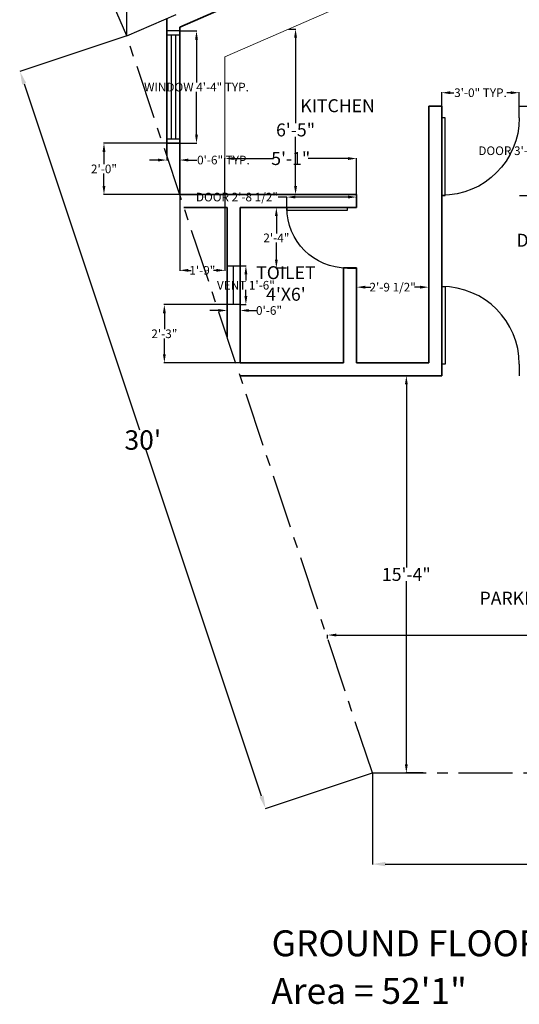
# Model space of a CAD drawing. Units: inches. Extents: x 1778 to 2384, y 384 to 1080.
# Tile 1 of 3: x 1778 to 2009, y 384 to 841. Entities that reach past the tile are written whole.
import ezdxf

# ---------------------------------------------------------------- set-up
doc = ezdxf.new("R2010")
doc.units = ezdxf.units.IN
doc.header["$MEASUREMENT"] = 0
doc.linetypes.add('CENTER', pattern=[2, 1.25, -0.25, 0.25, -0.25])
for name, color, linetype, lineweight in [('A-ANNO-DIMS', 2, 'Continuous', 18), ('A-ANNO-TEXT', 72, 'Continuous', 25), ('A-AREA-IDEN', 1, 'Continuous', 18), ('A-FLOR-FIXT', 8, 'Continuous', 18), ('A-GLAZ', 4, 'Continuous', 18), ('A-WALL', 7, 'Continuous', 35), ('C-PROP', 13, 'CENTER', 25), ('DOOR', 13, 'Continuous', 25)]:
    doc.layers.add(name, color=color, linetype=linetype, lineweight=lineweight)
doc.styles.get("Standard").update_dxf_attribs({"font": 'arial.ttf'})
doc.dimstyles.get("Standard").update_dxf_attribs({"dimtxt": 4, "dimasz": 4, "dimexe": 0.18, "dimexo": 0.0625, "dimgap": 0.09, "dimtad": 0, "dimtih": 1, "dimtoh": 1, "dimdec": 0, "dimzin": 0, "dimdsep": 46, "dimlunit": 3, "dimtxsty": 'Standard', "dimcen": 0.09, "dimadec": 0, "dimazin": 0, "dimtfac": 1, "dimtdec": 0, "dimtofl": 0, "dimtmove": 0, "dimatfit": 3, "dimfxl": 1, "dimtolj": 1, "dimtzin": 0, "dimarcsym": 0})

# ---------------------------------------------------------------- blocks, each defined once
blk = doc.blocks.new('*D2')
at = {"layer": 'A-ANNO-DIMS', "color": 0, "lineweight": -2, "transparency": 16777216}
for p, q in [((1941.36, 491.47), (1941.36, 449.11)), ((2181.36, 491.47), (2181.36, 449.11)), ((1947.36, 449.29), (2053.55, 449.29)), ((2175.36, 449.29), (2069.16, 449.29))]:
    blk.add_line(p, q, dxfattribs=at)
at = {"layer": 'A-ANNO-DIMS', "color": 0, "transparency": 16777216}
for points in [[(1947.36, 450.29), (1947.36, 448.29), (1941.36, 449.29)], [(2175.36, 450.29), (2175.36, 448.29), (2181.36, 449.29)]]:
    blk.add_solid(points, dxfattribs=at)
at = {"layer": 'Defpoints', "color": 0, "transparency": 16777216}
for p in [(1941.36, 491.53), (2181.36, 491.53), (2181.36, 449.29)]:
    blk.add_point(p, dxfattribs=at)
at = {"layer": 'A-ANNO-DIMS', "color": 0, "transparency": 16777216, "insert": (2061.36, 449.29), "char_height": 9, "attachment_point": 5}
blk.add_mtext("\\A1;20'", dxfattribs=at)
blk = doc.blocks.new('*D3')
at = {"layer": 'A-ANNO-DIMS', "color": 0, "lineweight": -2, "transparency": 16777216}
for p, q in [((1827.47, 833.04), (1777.86, 816.51)), ((1779.93, 810.88), (1833.39, 650.49)), ((1889.97, 480.73), (1836.51, 641.11)), ((1941.3, 491.51), (1891.69, 474.98))]:
    blk.add_line(p, q, dxfattribs=at)
at = {"layer": 'A-ANNO-DIMS', "color": 0, "transparency": 16777216}
for points in [[(1780.88, 811.19), (1778.98, 810.56), (1778.03, 816.57)], [(1890.91, 481.05), (1889.02, 480.41), (1891.86, 475.04)]]:
    blk.add_solid(points, dxfattribs=at)
at = {"layer": 'Defpoints', "color": 0, "transparency": 16777216}
for p in [(1827.53, 833.06), (1941.36, 491.53), (1891.86, 475.04)]:
    blk.add_point(p, dxfattribs=at)
at = {"layer": 'A-ANNO-DIMS', "color": 0, "transparency": 16777216, "insert": (1834.95, 645.8), "char_height": 9, "attachment_point": 5}
blk.add_mtext("\\A1;30'", dxfattribs=at)
blk = doc.blocks.new('*D4')
at = {"layer": 'A-ANNO-DIMS', "color": 0, "lineweight": -2, "transparency": 16777216}
for p, q in [((2238.23, 1077.18), (2031.58, 987.25)), ((2267.63, 1024.65), (2243.66, 1079.74)), ((1809.1, 890.44), (2015.76, 980.36)), ((1827.5, 833.12), (1803.53, 888.21))]:
    blk.add_line(p, q, dxfattribs=at)
at = {"layer": 'A-ANNO-DIMS', "color": 0, "transparency": 16777216}
for points in [[(2237.83, 1078.09), (2238.63, 1076.26), (2243.73, 1079.57)], [(1808.7, 891.35), (1809.5, 889.52), (1803.6, 888.04)]]:
    blk.add_solid(points, dxfattribs=at)
at = {"layer": 'Defpoints', "color": 0, "transparency": 16777216}
for p in [(2243.73, 1079.57), (2267.66, 1024.59), (1827.53, 833.06)]:
    blk.add_point(p, dxfattribs=at)
at = {"layer": 'A-ANNO-DIMS', "color": 0, "transparency": 16777216, "insert": (2023.67, 983.81), "char_height": 9, "attachment_point": 5}
blk.add_mtext("\\A1;40'", dxfattribs=at)
blk = doc.blocks.new('*D6')
at = {"layer": 'A-ANNO-DIMS', "color": 0, "lineweight": -2, "transparency": 16777216}
for p, q in [((1873.03, 759.6), (1873.03, 776.41)), ((1877.03, 776.23), (1895.47, 776.23)), ((1930.03, 776.23), (1911.6, 776.23)), ((1934.03, 759.6), (1934.03, 776.41))]:
    blk.add_line(p, q, dxfattribs=at)
at = {"layer": 'A-ANNO-DIMS', "color": 0, "transparency": 16777216}
for points in [[(1877.03, 776.89), (1877.03, 775.56), (1873.03, 776.23)], [(1930.03, 776.89), (1930.03, 775.56), (1934.03, 776.23)]]:
    blk.add_solid(points, dxfattribs=at)
at = {"layer": 'Defpoints', "color": 0, "transparency": 16777216}
for p in [(1934.03, 776.23), (1873.03, 759.53), (1934.03, 759.53)]:
    blk.add_point(p, dxfattribs=at)
at = {"layer": 'A-ANNO-DIMS', "color": 0, "transparency": 16777216, "insert": (1903.53, 776.23), "char_height": 6, "attachment_point": 5}
blk.add_mtext('\\A1;5\'-1"', dxfattribs=at)
blk = doc.blocks.new('*D8')
at = {"layer": 'A-ANNO-DIMS', "color": 0, "lineweight": -2, "transparency": 16777216}
for p, q in [((1964.93, 675.53), (1956.93, 675.53)), ((1957.11, 671.53), (1957.11, 586.69)), ((1957.11, 495.53), (1957.11, 580.38)), ((1964.93, 491.53), (1956.93, 491.53))]:
    blk.add_line(p, q, dxfattribs=at)
at = {"layer": 'A-ANNO-DIMS', "color": 0, "transparency": 16777216}
for points in [[(1956.44, 671.53), (1957.78, 671.53), (1957.11, 675.53)], [(1956.44, 495.53), (1957.78, 495.53), (1957.11, 491.53)]]:
    blk.add_solid(points, dxfattribs=at)
at = {"layer": 'Defpoints', "color": 0, "transparency": 16777216}
for p in [(1957.11, 675.53), (1964.99, 675.53), (1964.99, 491.53)]:
    blk.add_point(p, dxfattribs=at)
at = {"layer": 'A-ANNO-DIMS', "color": 0, "transparency": 16777216, "insert": (1957.11, 583.53), "char_height": 6, "attachment_point": 5}
blk.add_mtext('\\A1;15\'-4"', dxfattribs=at)
blk = doc.blocks.new('*D9')
at = {"layer": 'A-ANNO-DIMS', "color": 0, "lineweight": -2, "transparency": 16777216}
for p, q in [((1920.61, 553.84), (1920.61, 555.61)), ((1924.61, 555.43), (2045.38, 555.43)), ((2187.04, 555.43), (2066.27, 555.43)), ((2191.04, 551.41), (2191.04, 555.61))]:
    blk.add_line(p, q, dxfattribs=at)
at = {"layer": 'A-ANNO-DIMS', "color": 0, "transparency": 16777216}
for points in [[(1924.61, 556.1), (1924.61, 554.77), (1920.61, 555.43)], [(2187.04, 556.1), (2187.04, 554.77), (2191.04, 555.43)]]:
    blk.add_solid(points, dxfattribs=at)
at = {"layer": 'Defpoints', "color": 0, "transparency": 16777216}
for p in [(1920.61, 555.43), (1920.61, 553.77), (2191.04, 551.35)]:
    blk.add_point(p, dxfattribs=at)
at = {"layer": 'A-ANNO-DIMS', "color": 0, "transparency": 16777216, "insert": (2055.83, 555.43), "char_height": 6, "attachment_point": 5}
blk.add_mtext('\\A1;22\'-6"', dxfattribs=at)
blk = doc.blocks.new('*D11')
at = {"layer": 'A-ANNO-DIMS', "color": 0, "lineweight": -2, "transparency": 16777216}
for p, q in [((1902.55, 836.24), (1905.94, 836.24)), ((1905.76, 832.24), (1905.76, 792.65)), ((1905.76, 763.53), (1905.76, 786.34)), ((1902.55, 759.53), (1905.94, 759.53))]:
    blk.add_line(p, q, dxfattribs=at)
at = {"layer": 'A-ANNO-DIMS', "color": 0, "transparency": 16777216}
for points in [[(1905.09, 832.24), (1906.42, 832.24), (1905.76, 836.24)], [(1905.09, 763.53), (1906.42, 763.53), (1905.76, 759.53)]]:
    blk.add_solid(points, dxfattribs=at)
at = {"layer": 'Defpoints', "color": 0, "transparency": 16777216}
for p in [(1902.48, 836.24), (1902.48, 759.53), (1905.76, 759.53)]:
    blk.add_point(p, dxfattribs=at)
at = {"layer": 'A-ANNO-DIMS', "color": 0, "transparency": 16777216, "insert": (1905.76, 789.49), "char_height": 6, "attachment_point": 5}
blk.add_mtext('\\A1;6\'-5"', dxfattribs=at)
blk = doc.blocks.new('*U14')
for p, q in [((0, 0), (0, -6)), ((40, 0), (40, -6))]:
    blk.add_line(p, q)
blk.add_lwpolyline([(0, 0), (0, 40), (1.75, 40), (1.75, 0)], close=True)
blk.add_arc((0, 0), 40, 0, 90)
blk = doc.blocks.new('DOOR')
blk.add_blockref('*U14', (1810.9, 983.44))
blk = doc.blocks.new('WINDOW')
for p, q in [((1664.47, 998.33), (1658.47, 998.33)), ((1658.47, 950.33), (1664.47, 950.33))]:
    blk.add_line(p, q)
at = {"layer": 'DOOR'}
for p, q in [((1664.47, 1000.33), (1658.47, 1000.33)), ((1660.47, 998.33), (1660.47, 950.33)), ((1662.47, 998.33), (1662.47, 950.33)), ((1658.47, 948.33), (1664.47, 948.33))]:
    blk.add_line(p, q, dxfattribs=at)
blk = doc.blocks.new('WIN')
at = {"layer": 'Defpoints'}
for p, q in [((1658.47, 1000.33), (1658.47, 948.33)), ((1664.47, 1000.33), (1664.47, 948.33))]:
    blk.add_line(p, q, dxfattribs=at)
at = {"layer": 'DOOR'}
blk.add_blockref('WINDOW', (0, 0), dxfattribs=at)
blk = doc.blocks.new('VENTILATION')
at = {"layer": 'Defpoints'}
for p, q in [((1829.39, 697.16), (1829.39, 715.16)), ((1835.39, 715.16), (1835.39, 697.16))]:
    blk.add_line(p, q, dxfattribs=at)
at = {"layer": 'DOOR'}
for p, q in [((1829.39, 715.16), (1835.39, 715.16)), ((1832.39, 697.16), (1832.39, 715.16)), ((1835.39, 697.16), (1829.39, 697.16))]:
    blk.add_line(p, q, dxfattribs=at)
blk = doc.blocks.new('*D21')
at = {"layer": 'A-ANNO-DIMS', "color": 0, "lineweight": -2, "transparency": 16777216}
for p, q in [((2009.54, 800.53), (2015.86, 800.53)), ((2015.68, 796.53), (2015.68, 782.01)), ((2015.68, 763.16), (2015.68, 777.68)), ((2009.54, 759.16), (2015.86, 759.16))]:
    blk.add_line(p, q, dxfattribs=at)
at = {"layer": 'A-ANNO-DIMS', "color": 0, "transparency": 16777216}
for points in [[(2015.01, 796.53), (2016.35, 796.53), (2015.68, 800.53)], [(2015.01, 763.16), (2016.35, 763.16), (2015.68, 759.16)]]:
    blk.add_solid(points, dxfattribs=at)
at = {"layer": 'Defpoints', "color": 0, "transparency": 16777216}
for p in [(2009.47, 800.53), (2009.47, 759.16), (2015.68, 759.16)]:
    blk.add_point(p, dxfattribs=at)
at = {"layer": 'A-ANNO-DIMS', "color": 0, "transparency": 16777216, "insert": (2015.68, 779.85), "char_height": 4, "attachment_point": 5}
blk.add_mtext('\\A1;DOOR 3\'-5 1/2" TYP.', dxfattribs=at)
blk = doc.blocks.new('*D22')
at = {"layer": 'A-ANNO-DIMS', "color": 0, "lineweight": -2, "transparency": 16777216}
for p, q in [((1973.49, 800.6), (1973.49, 806.92)), ((1977.49, 806.74), (1979.2, 806.74)), ((2005.47, 806.74), (2003.76, 806.74)), ((2009.47, 800.6), (2009.47, 806.92))]:
    blk.add_line(p, q, dxfattribs=at)
at = {"layer": 'A-ANNO-DIMS', "color": 0, "transparency": 16777216}
for points in [[(1977.49, 807.41), (1977.49, 806.07), (1973.49, 806.74)], [(2005.47, 807.41), (2005.47, 806.07), (2009.47, 806.74)]]:
    blk.add_solid(points, dxfattribs=at)
at = {"layer": 'Defpoints', "color": 0, "transparency": 16777216}
for p in [(2009.47, 806.74), (1973.49, 800.53), (2009.47, 800.53)]:
    blk.add_point(p, dxfattribs=at)
at = {"layer": 'A-ANNO-DIMS', "color": 0, "transparency": 16777216, "insert": (1991.48, 806.74), "char_height": 4, "attachment_point": 5}
blk.add_mtext('\\A1;3\'-0" TYP.', dxfattribs=at)
blk = doc.blocks.new('*D27')
at = {"layer": 'A-ANNO-DIMS', "color": 0, "lineweight": -2, "transparency": 16777216}
for p, q in [((1901.7, 758.38), (1897.7, 758.38)), ((1901.7, 753.6), (1901.7, 758.56)), ((1930.03, 758.38), (1905.7, 758.38)), ((1934.03, 753.6), (1934.03, 758.56))]:
    blk.add_line(p, q, dxfattribs=at)
at = {"layer": 'A-ANNO-DIMS', "color": 0, "transparency": 16777216}
for points in [[(1905.7, 759.05), (1905.7, 757.72), (1901.7, 758.38)], [(1930.03, 759.05), (1930.03, 757.72), (1934.03, 758.38)]]:
    blk.add_solid(points, dxfattribs=at)
at = {"layer": 'Defpoints', "color": 0, "transparency": 16777216}
for p in [(1901.7, 758.38), (1901.7, 753.53), (1934.03, 753.53)]:
    blk.add_point(p, dxfattribs=at)
at = {"layer": 'A-ANNO-DIMS', "color": 0, "transparency": 16777216, "insert": (1878.57, 758.38), "char_height": 4, "attachment_point": 5}
blk.add_mtext('\\A1;DOOR 2\'-8 1/2"', dxfattribs=at)
blk = doc.blocks.new('*D28')
at = {"layer": 'A-ANNO-DIMS', "color": 0, "lineweight": -2, "transparency": 16777216}
for p, q in [((1901.63, 753.53), (1896.67, 753.53)), ((1896.85, 749.53), (1896.85, 741.57)), ((1896.85, 729.41), (1896.85, 737.38)), ((1901.63, 725.41), (1896.67, 725.41))]:
    blk.add_line(p, q, dxfattribs=at)
at = {"layer": 'A-ANNO-DIMS', "color": 0, "transparency": 16777216}
for points in [[(1896.18, 749.53), (1897.51, 749.53), (1896.85, 753.53)], [(1896.18, 729.41), (1897.51, 729.41), (1896.85, 725.41)]]:
    blk.add_solid(points, dxfattribs=at)
at = {"layer": 'Defpoints', "color": 0, "transparency": 16777216}
for p in [(1901.7, 753.53), (1896.85, 725.41), (1901.7, 725.41)]:
    blk.add_point(p, dxfattribs=at)
at = {"layer": 'A-ANNO-DIMS', "color": 0, "transparency": 16777216, "insert": (1896.85, 739.47), "char_height": 4, "attachment_point": 5}
blk.add_mtext('\\A1;2\'-4"', dxfattribs=at)
blk = doc.blocks.new('*D29')
at = {"layer": 'A-ANNO-DIMS', "color": 0, "lineweight": -2, "transparency": 16777216}
for p, q in [((1852.1, 835.33), (1860.01, 835.33)), ((1859.83, 831.33), (1859.83, 811.49)), ((1859.83, 787.33), (1859.83, 807.17)), ((1852.1, 783.33), (1860.01, 783.33))]:
    blk.add_line(p, q, dxfattribs=at)
at = {"layer": 'A-ANNO-DIMS', "color": 0, "transparency": 16777216}
for points in [[(1859.17, 831.33), (1860.5, 831.33), (1859.83, 835.33)], [(1859.17, 787.33), (1860.5, 787.33), (1859.83, 783.33)]]:
    blk.add_solid(points, dxfattribs=at)
at = {"layer": 'Defpoints', "color": 0, "transparency": 16777216}
for p in [(1852.03, 835.33), (1859.83, 835.33), (1852.03, 783.33)]:
    blk.add_point(p, dxfattribs=at)
at = {"layer": 'A-ANNO-DIMS', "color": 0, "transparency": 16777216, "insert": (1859.83, 809.33), "char_height": 4, "attachment_point": 5}
blk.add_mtext('\\A1;WINDOW 4\'-4" TYP.', dxfattribs=at)
blk = doc.blocks.new('*D30')
at = {"layer": 'A-ANNO-DIMS', "color": 0, "lineweight": -2, "transparency": 16777216}
for p, q in [((1846.03, 783.26), (1846.03, 775.35)), ((1852.03, 783.26), (1852.03, 775.35)), ((1842.03, 775.53), (1838.03, 775.53)), ((1856.03, 775.53), (1860.03, 775.53))]:
    blk.add_line(p, q, dxfattribs=at)
at = {"layer": 'A-ANNO-DIMS', "color": 0, "transparency": 16777216}
for points in [[(1842.03, 776.19), (1842.03, 774.86), (1846.03, 775.53)], [(1856.03, 776.19), (1856.03, 774.86), (1852.03, 775.53)]]:
    blk.add_solid(points, dxfattribs=at)
at = {"layer": 'Defpoints', "color": 0, "transparency": 16777216}
for p in [(1846.03, 783.33), (1852.03, 783.33), (1852.03, 775.53)]:
    blk.add_point(p, dxfattribs=at)
at = {"layer": 'A-ANNO-DIMS', "color": 0, "transparency": 16777216, "insert": (1872.31, 775.53), "char_height": 4, "attachment_point": 5}
blk.add_mtext('\\A1;0\'-6" TYP.', dxfattribs=at)
blk = doc.blocks.new('*D31')
at = {"layer": 'A-ANNO-DIMS', "color": 0, "lineweight": -2, "transparency": 16777216}
for p, q in [((1880.09, 726.53), (1882.91, 726.53)), ((1882.73, 722.53), (1882.73, 719.67)), ((1882.73, 712.53), (1882.73, 715.4)), ((1880.09, 708.53), (1882.91, 708.53))]:
    blk.add_line(p, q, dxfattribs=at)
at = {"layer": 'A-ANNO-DIMS', "color": 0, "transparency": 16777216}
for points in [[(1882.06, 722.53), (1883.4, 722.53), (1882.73, 726.53)], [(1882.06, 712.53), (1883.4, 712.53), (1882.73, 708.53)]]:
    blk.add_solid(points, dxfattribs=at)
at = {"layer": 'Defpoints', "color": 0, "transparency": 16777216}
for p in [(1880.03, 726.53), (1882.73, 726.53), (1880.03, 708.53)]:
    blk.add_point(p, dxfattribs=at)
at = {"layer": 'A-ANNO-DIMS', "color": 0, "transparency": 16777216, "insert": (1882.73, 717.53), "char_height": 4, "attachment_point": 5}
blk.add_mtext('\\A1;VENT 1\'-6"', dxfattribs=at)
blk = doc.blocks.new('*D32')
at = {"layer": 'A-ANNO-DIMS', "color": 0, "lineweight": -2, "transparency": 16777216}
for p, q in [((1874.03, 708.47), (1874.03, 705.65)), ((1880.03, 708.47), (1880.03, 705.65)), ((1870.03, 705.83), (1866.03, 705.83)), ((1884.03, 705.83), (1888.03, 705.83))]:
    blk.add_line(p, q, dxfattribs=at)
at = {"layer": 'A-ANNO-DIMS', "color": 0, "transparency": 16777216}
for points in [[(1870.03, 706.5), (1870.03, 705.17), (1874.03, 705.83)], [(1884.03, 706.5), (1884.03, 705.17), (1880.03, 705.83)]]:
    blk.add_solid(points, dxfattribs=at)
at = {"layer": 'Defpoints', "color": 0, "transparency": 16777216}
for p in [(1874.03, 708.53), (1880.03, 708.53), (1880.03, 705.83)]:
    blk.add_point(p, dxfattribs=at)
at = {"layer": 'A-ANNO-DIMS', "color": 0, "transparency": 16777216, "insert": (1893.44, 705.83), "char_height": 4, "attachment_point": 5}
blk.add_mtext('\\A1;0\'-6"', dxfattribs=at)
blk = doc.blocks.new('*D36')
at = {"layer": 'A-ANNO-DIMS', "color": 0, "lineweight": -2, "transparency": 16777216}
for p, q in [((1827.53, 833.13), (1827.53, 1059.87)), ((1831.53, 1059.69), (2040.63, 1059.69)), ((2263.66, 1059.69), (2054.55, 1059.69)), ((2267.66, 1024.66), (2267.66, 1059.87))]:
    blk.add_line(p, q, dxfattribs=at)
at = {"layer": 'A-ANNO-DIMS', "color": 0, "transparency": 16777216}
for points in [[(1831.53, 1060.36), (1831.53, 1059.03), (1827.53, 1059.69)], [(2263.66, 1060.36), (2263.66, 1059.03), (2267.66, 1059.69)]]:
    blk.add_solid(points, dxfattribs=at)
at = {"layer": 'Defpoints', "color": 0, "transparency": 16777216}
for p in [(2267.66, 1059.69), (2267.66, 1024.59), (1827.53, 833.06)]:
    blk.add_point(p, dxfattribs=at)
at = {"layer": 'A-ANNO-DIMS', "color": 0, "transparency": 16777216, "insert": (2047.59, 1059.69), "char_height": 4, "attachment_point": 5}
blk.add_mtext('\\A1;36\'-8"', dxfattribs=at)
blk = doc.blocks.new('*D42')
at = {"layer": 'A-ANNO-DIMS', "color": 0, "lineweight": -2, "transparency": 16777216}
for p, q in [((1851.97, 783.33), (1816.75, 783.33)), ((1816.93, 779.33), (1816.93, 773.56)), ((1816.93, 763.53), (1816.93, 769.3)), ((1851.97, 759.53), (1816.75, 759.53))]:
    blk.add_line(p, q, dxfattribs=at)
at = {"layer": 'A-ANNO-DIMS', "color": 0, "transparency": 16777216}
for points in [[(1816.27, 779.33), (1817.6, 779.33), (1816.93, 783.33)], [(1816.27, 763.53), (1817.6, 763.53), (1816.93, 759.53)]]:
    blk.add_solid(points, dxfattribs=at)
at = {"layer": 'Defpoints', "color": 0, "transparency": 16777216}
for p in [(1816.93, 783.33), (1852.03, 783.33), (1852.03, 759.53)]:
    blk.add_point(p, dxfattribs=at)
at = {"layer": 'A-ANNO-DIMS', "color": 0, "transparency": 16777216, "insert": (1816.93, 771.43), "char_height": 4, "attachment_point": 5}
blk.add_mtext('\\A1;2\'-0"', dxfattribs=at)
blk = doc.blocks.new('*D43')
at = {"layer": 'A-ANNO-DIMS', "color": 0, "lineweight": -2, "transparency": 16777216}
for p, q in [((1879.97, 708.53), (1844.75, 708.53)), ((1844.93, 704.53), (1844.93, 697.17)), ((1844.93, 685.53), (1844.93, 692.9)), ((1879.97, 681.53), (1844.75, 681.53))]:
    blk.add_line(p, q, dxfattribs=at)
at = {"layer": 'A-ANNO-DIMS', "color": 0, "transparency": 16777216}
for points in [[(1844.26, 704.53), (1845.6, 704.53), (1844.93, 708.53)], [(1844.26, 685.53), (1845.6, 685.53), (1844.93, 681.53)]]:
    blk.add_solid(points, dxfattribs=at)
at = {"layer": 'Defpoints', "color": 0, "transparency": 16777216}
for p in [(1844.93, 708.53), (1880.03, 708.53), (1880.03, 681.53)]:
    blk.add_point(p, dxfattribs=at)
at = {"layer": 'A-ANNO-DIMS', "color": 0, "transparency": 16777216, "insert": (1844.93, 695.03), "char_height": 4, "attachment_point": 5}
blk.add_mtext('\\A1;2\'-3"', dxfattribs=at)
blk = doc.blocks.new('*D44')
at = {"layer": 'A-ANNO-DIMS', "color": 0, "lineweight": -2, "transparency": 16777216}
for p, q in [((1934.03, 681.6), (1934.03, 716.81)), ((1938.03, 716.63), (1940.66, 716.63)), ((1963.49, 716.63), (1960.86, 716.63)), ((1967.49, 681.6), (1967.49, 716.81))]:
    blk.add_line(p, q, dxfattribs=at)
at = {"layer": 'A-ANNO-DIMS', "color": 0, "transparency": 16777216}
for points in [[(1938.03, 717.3), (1938.03, 715.97), (1934.03, 716.63)], [(1963.49, 717.3), (1963.49, 715.97), (1967.49, 716.63)]]:
    blk.add_solid(points, dxfattribs=at)
at = {"layer": 'Defpoints', "color": 0, "transparency": 16777216}
for p in [(1967.49, 716.63), (1934.03, 681.53), (1967.49, 681.53)]:
    blk.add_point(p, dxfattribs=at)
at = {"layer": 'A-ANNO-DIMS', "color": 0, "transparency": 16777216, "insert": (1950.76, 716.63), "char_height": 4, "attachment_point": 5}
blk.add_mtext('\\A1;2\'-9 1/2"', dxfattribs=at)
blk = doc.blocks.new('*D45')
at = {"layer": 'A-ANNO-DIMS', "color": 0, "lineweight": -2, "transparency": 16777216}
for p, q in [((1852.03, 759.47), (1852.03, 724.25)), ((1873.03, 759.47), (1873.03, 724.25)), ((1856.03, 724.43), (1857.32, 724.43)), ((1869.03, 724.43), (1867.75, 724.43))]:
    blk.add_line(p, q, dxfattribs=at)
at = {"layer": 'A-ANNO-DIMS', "color": 0, "transparency": 16777216}
for points in [[(1856.03, 725.1), (1856.03, 723.77), (1852.03, 724.43)], [(1869.03, 725.1), (1869.03, 723.77), (1873.03, 724.43)]]:
    blk.add_solid(points, dxfattribs=at)
at = {"layer": 'Defpoints', "color": 0, "transparency": 16777216}
for p in [(1852.03, 759.53), (1873.03, 759.53), (1852.03, 724.43)]:
    blk.add_point(p, dxfattribs=at)
at = {"layer": 'A-ANNO-DIMS', "color": 0, "transparency": 16777216, "insert": (1862.53, 724.43), "char_height": 4, "attachment_point": 5}
blk.add_mtext('\\A1;1\'-9"', dxfattribs=at)

msp = doc.modelspace()

# ---------------------------------------------------------------- linework, layer by layer
at = {"layer": 'A-FLOR-FIXT', "ltscale": 20}
msp.add_line((1873.03, 823.42), (1940.03, 852.58), dxfattribs=at)
at = {"layer": 'A-FLOR-FIXT'}
msp.add_line((1873.03, 759.53), (1873.03, 823.42), dxfattribs=at)
at = {"layer": 'A-WALL', "ltscale": 20}
for p, q in [((1852.03, 837.18), (2092.89, 942)), ((1967.49, 800.53), (1973.49, 800.53)), ((1852.03, 759.53), (1934.03, 759.53)), ((1854.03, 753.53), (1874.03, 753.53)), ((1880.03, 753.53), (1934.03, 753.53)), ((1880.03, 681.53), (1928.03, 681.53)), ((1934.03, 681.53), (1967.49, 681.53)), ((1940.03, 681.53), (1967.49, 681.53)), ((1880.03, 675.53), (1973.49, 675.53))]:
    msp.add_line(p, q, dxfattribs=at)
at = {"layer": 'A-WALL'}
for p, q in [((1846.03, 777.54), (1846.03, 841.12)), ((1852.03, 759.53), (1852.03, 837.18)), ((1967.49, 681.53), (1967.49, 800.53)), ((1973.49, 675.53), (1973.49, 800.53)), ((1934.03, 753.53), (1934.03, 759.53)), ((1874.03, 693.53), (1874.03, 753.53)), ((1880.03, 681.53), (1880.03, 753.53)), ((1928.03, 681.53), (1928.03, 725.53)), ((1928.03, 725.53), (1934.03, 725.53)), ((1934.03, 681.53), (1934.03, 725.53))]:
    msp.add_line(p, q, dxfattribs=at)
at = {"layer": 'C-PROP', "ltscale": 20}
for p, q in [((1827.53, 833.06), (2267.66, 1024.59)), ((1941.36, 491.53), (1827.53, 833.06)), ((1941.36, 491.53), (2181.36, 491.53))]:
    msp.add_line(p, q, dxfattribs=at)

# ---------------------------------------------------------------- block references
at = {"layer": 'A-GLAZ'}
for name, p in [('WIN', (187.56, -165)), ('VENTILATION', (44.64, 11.37))]:
    msp.add_blockref(name, p, dxfattribs=at)
at = {"layer": 'DOOR'}
for p, xscale, yscale, zscale, rotation in [((344.59, 1679.74), -0.8994999112294854, 0.8994999112294854, 0.8994999112294854, 180), ((2621.14, 2026.54), -0.7029690829752921, 0.7029690829752921, 0.7029690829752921, 90)]:
    msp.add_blockref('DOOR', p, dxfattribs=dict(at, xscale=xscale, yscale=yscale, zscale=zscale, rotation=rotation))
at = {"layer": 'DOOR', "xscale": 0.8994117399316744, "yscale": 0.8994117399316744, "zscale": 0.8994117399316744}
msp.add_blockref('DOOR', (344.75, -203.59), dxfattribs=at)

# ---------------------------------------------------------------- texts
at = {"layer": 'A-ANNO-TEXT', "char_height": 12, "attachment_point": 1}
for s, width, insert in [('GROUND FLOOR ARCHITECTURAL PLAN', 680.8928, (1894.65, 418.6)), ('Area = 52\'1"', 279.3768, (1894.56, 396.54))]:
    msp.add_mtext_dynamic_manual_height_columns(s, width=width, gutter_width=1, heights=[0], dxfattribs=dict(at, insert=insert))
at = {"layer": 'A-AREA-IDEN', "char_height": 6}
for s, width, insert, attachment_point in [('KITCHEN', 72.6444, (1907.98, 803.71), 1), ('DRAWING ROOM\\P10\'X9\'5"', 72.6444, (2039.54, 741.37), 2), ("TOILET\\P4'X6'", 36.3222, (1901.28, 726.35), 2), ('PARKING', 72.6444, (2008.36, 575.52), 2)]:
    msp.add_mtext_dynamic_manual_height_columns(s, width=width, gutter_width=1, heights=[0], dxfattribs=dict(at, insert=insert, attachment_point=attachment_point))

# ---------------------------------------------------------------- dimensions: what is measured, and where the dimension line sits
at = {"layer": 'A-ANNO-DIMS'}
for p1, p2, distance, picture, middle in [((1827.53, 833.06), (2267.66, 1024.59), 59.96, '*D4', (2023.67, 983.81)), ((1827.53, 833.06), (1941.36, 491.53), -52.17, '*D3', (1834.95, 645.8)), ((1941.36, 491.53), (2181.36, 491.53), -42.24, '*D2', (2061.36, 449.29))]:
    dim = msp.add_aligned_dim(p1=p1, p2=p2, distance=distance, dimstyle='Standard', override={"dimtxt": 9, "dimasz": 6, "dimclrd": 0, "dimclre": 0, "dimclrt": 0}, dxfattribs=at)
    dim.commit()
    dim.dimension.update_dxf_attribs({"geometry": picture, "text_midpoint": middle})
for base, p1, p2, override, picture, middle in [((2267.66, 1059.69), (1827.53, 833.06), (2267.66, 1024.59), {"dimdec": 1, "dimlfac": 1, "dimrnd": 0, "dimzin": 1, "dimdsep": 46, "dimlunit": 4, "dimfrac": 2}, '*D36', (2047.59, 1059.69)), ((1934.03, 776.23), (1873.03, 759.53), (1934.03, 759.53), {"dimtxt": 6, "dimclrd": 0, "dimclre": 0, "dimclrt": 0}, '*D6', (1903.53, 776.23)), ((1967.49, 716.63), (1934.03, 681.53), (1967.49, 681.53), {"dimdec": 1, "dimlfac": 1, "dimrnd": 0, "dimzin": 1, "dimdsep": 46, "dimlunit": 4, "dimfrac": 2}, '*D44', (1950.76, 716.63)), ((1880.03, 705.83), (1874.03, 708.53), (1880.03, 708.53), {"dimdec": 1, "dimlfac": 1, "dimrnd": 0, "dimzin": 1, "dimdsep": 46, "dimlunit": 4, "dimfrac": 2}, '*D32', (1893.44, 705.83)), ((1920.61, 555.43), (2191.04, 551.35), (1920.61, 553.77), {"dimtxt": 6, "dimclrd": 0, "dimclre": 0, "dimclrt": 0}, '*D9', (2055.83, 555.43))]:
    dim = msp.add_linear_dim(base=base, p1=p1, p2=p2, dimstyle='Standard', override=override, dxfattribs=at)
    dim.commit()
    dim.dimension.update_dxf_attribs({"geometry": picture, "text_midpoint": middle})
for base, p1, p2, angle, text, picture, middle in [((1859.83, 835.33), (1852.03, 783.33), (1852.03, 835.33), 90, 'WINDOW <> TYP.', '*D29', (1859.83, 809.33)), ((2015.68, 759.16), (2009.47, 800.53), (2009.47, 759.16), 270, 'DOOR <> TYP.', '*D21', (2015.68, 779.85)), ((1901.7, 758.38), (1934.03, 753.53), (1901.7, 753.53), 180, 'DOOR <>', '*D27', (1878.57, 758.38)), ((1882.73, 726.53), (1880.03, 708.53), (1880.03, 726.53), 90, 'VENT <>', '*D31', (1882.73, 717.53))]:
    dim = msp.add_linear_dim(base=base, p1=p1, p2=p2, angle=angle, text=text, dimstyle='Standard', override={"dimdec": 1, "dimlfac": 1, "dimrnd": 0, "dimzin": 1, "dimdsep": 46, "dimlunit": 4, "dimfrac": 2}, dxfattribs=at)
    dim.commit()
    dim.dimension.update_dxf_attribs({"geometry": picture, "text_midpoint": middle})
dim = msp.add_linear_dim(base=(1905.76, 759.53), p1=(1902.48, 836.24), p2=(1902.48, 759.53), angle=90, dimstyle='Standard', override={"dimtxt": 6, "dimclrd": 0, "dimclre": 0, "dimclrt": 0}, dxfattribs=at)
dim.commit()
dim.dimension.update_dxf_attribs({"geometry": '*D11', "text_midpoint": (1905.76, 789.49), "dimtype": 160})
for base, p1, p2, picture, middle in [((2009.47, 806.74), (1973.49, 800.53), (2009.47, 800.53), '*D22', (1991.48, 806.74)), ((1852.03, 775.53), (1846.03, 783.33), (1852.03, 783.33), '*D30', (1872.31, 775.53))]:
    dim = msp.add_linear_dim(base=base, p1=p1, p2=p2, text='<> TYP.', dimstyle='Standard', override={"dimdec": 1, "dimlfac": 1, "dimrnd": 0, "dimzin": 1, "dimdsep": 46, "dimlunit": 4, "dimfrac": 2}, dxfattribs=at)
    dim.commit()
    dim.dimension.update_dxf_attribs({"geometry": picture, "text_midpoint": middle})
for base, p1, p2, angle, override, picture, middle in [((1816.93, 783.33), (1852.03, 759.53), (1852.03, 783.33), 90, {"dimdec": 1, "dimlfac": 1, "dimrnd": 0, "dimzin": 1, "dimdsep": 46, "dimlunit": 4, "dimfrac": 2}, '*D42', (1816.93, 771.43)), ((1852.03, 724.43), (1873.03, 759.53), (1852.03, 759.53), 180, {"dimdec": 1, "dimlfac": 1, "dimrnd": 0, "dimzin": 1, "dimdsep": 46, "dimlunit": 4, "dimfrac": 2}, '*D45', (1862.53, 724.43)), ((1896.85, 725.41), (1901.7, 753.53), (1901.7, 725.41), 270, {"dimdec": 1, "dimlfac": 1, "dimrnd": 0, "dimzin": 1, "dimdsep": 46, "dimlunit": 4, "dimfrac": 2}, '*D28', (1896.85, 739.47)), ((1844.93, 708.53), (1880.03, 681.53), (1880.03, 708.53), 90, {"dimdec": 1, "dimlfac": 1, "dimrnd": 0, "dimzin": 1, "dimdsep": 46, "dimlunit": 4, "dimfrac": 2}, '*D43', (1844.93, 695.03)), ((1957.11, 675.53), (1964.99, 491.53), (1964.99, 675.53), 90, {"dimtxt": 6, "dimclrd": 0, "dimclre": 0, "dimclrt": 0}, '*D8', (1957.11, 583.53))]:
    dim = msp.add_linear_dim(base=base, p1=p1, p2=p2, angle=angle, dimstyle='Standard', override=override, dxfattribs=at)
    dim.commit()
    dim.dimension.update_dxf_attribs({"geometry": picture, "text_midpoint": middle})

doc.saveas('drawing.dxf')
